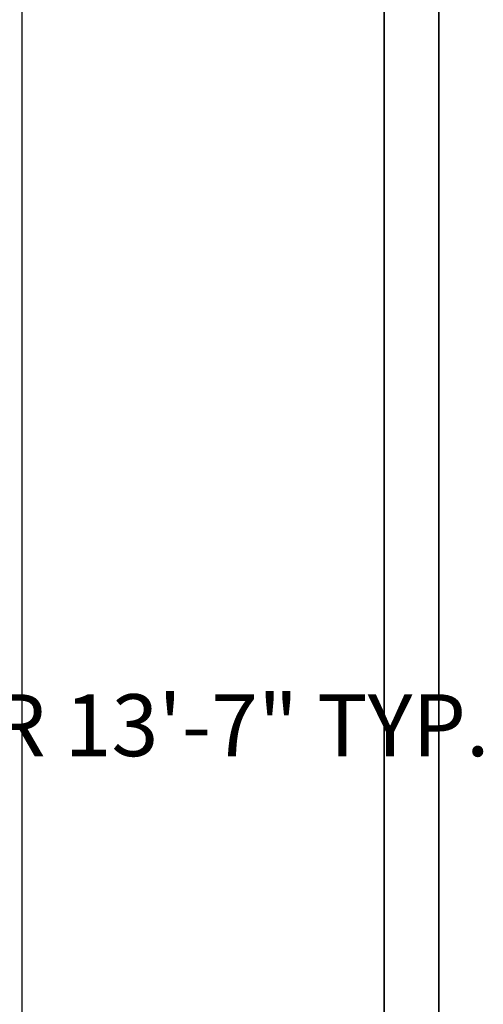
# Model space of a CAD drawing. Units: inches. Extents: x 1077 to 2505, y 1892 to 2728.
# Tile 10 of 26: x 1579 to 1655, y 2176 to 2338. Entities that reach past the tile are written whole.
import ezdxf

# ---------------------------------------------------------------- set-up
doc = ezdxf.new("R2010")
doc.units = ezdxf.units.IN
doc.linetypes.add('ACAD_ISO02W100', pattern=[15, 12, -3])
doc.layers.get('Defpoints').update_dxf_attribs({"color": 220, "linetype": 'ACAD_ISO02W100'})
doc.layers.add('A-ANNO-DIMS', color=2, linetype='Continuous', lineweight=18)
doc.layers.add('A-ANNO-TTLB', color=7, linetype='Continuous', lineweight=35)
doc.styles.get("Standard").update_dxf_attribs({"font": 'arial.ttf'})
doc.dimstyles.get("Standard").update_dxf_attribs({"dimtxt": 10.18, "dimasz": 0.18, "dimexe": 0.18, "dimexo": 0.0625, "dimgap": 0.09, "dimtad": 0, "dimtih": 1, "dimtoh": 1, "dimdec": 0, "dimzin": 0, "dimdsep": 46, "dimlunit": 3, "dimtxsty": 'Standard', "dimcen": 0.09, "dimadec": 0, "dimazin": 0, "dimtfac": 1, "dimtdec": 0, "dimtofl": 0, "dimtmove": 0, "dimatfit": 3, "dimfxl": 1, "dimtolj": 1, "dimtzin": 0, "dimarcsym": 0})

# ---------------------------------------------------------------- blocks, each defined once
blk = doc.blocks.new('*D14')
at = {"layer": 'A-ANNO-DIMS', "color": 0, "lineweight": -2, "transparency": 16777216}
for p, q in [((1555.59, 2651.66), (1579.43, 2651.66)), ((1579.25, 2651.48), (1579.25, 2375.3)), ((1579.25, 2088.54), (1579.25, 2364.72)), ((1555.59, 2088.36), (1579.43, 2088.36))]:
    blk.add_line(p, q, dxfattribs=at)
at = {"layer": 'A-ANNO-DIMS', "color": 0, "transparency": 16777216}
for points in [[(1579.22, 2651.48), (1579.28, 2651.48), (1579.25, 2651.66)], [(1579.22, 2088.54), (1579.28, 2088.54), (1579.25, 2088.36)]]:
    blk.add_solid(points, dxfattribs=at)
at = {"layer": 'Defpoints', "color": 0, "transparency": 16777216}
for p in [(1555.53, 2651.66), (1555.53, 2088.36), (1579.25, 2088.36)]:
    blk.add_point(p, dxfattribs=at)
at = {"layer": 'A-ANNO-DIMS', "color": 0, "transparency": 16777216, "insert": (1579.25, 2370.01), "char_height": 10.18, "attachment_point": 5}
blk.add_mtext('\\A1;46\'-11"', dxfattribs=at)
blk = doc.blocks.new('SHEET-FRAME-RESIDENTIAL')
for points in [[(0, 830.04), (543.52, 830.04), (543.52, 0), (0, 0)], [(9, 821.04), (534.52, 821.04), (534.52, 9), (9, 9)]]:
    blk.add_lwpolyline(points, close=True)
blk = doc.blocks.new('*D44')
at = {"layer": 'A-ANNO-DIMS', "color": 0, "lineweight": -2, "transparency": 16777216}
for p, q in [((1547.59, 2303.16), (1572.17, 2303.16)), ((1571.99, 2302.98), (1571.99, 2226.98)), ((1571.99, 2140.26), (1571.99, 2216.26)), ((1547.59, 2140.08), (1572.17, 2140.08))]:
    blk.add_line(p, q, dxfattribs=at)
at = {"layer": 'A-ANNO-DIMS', "color": 0, "transparency": 16777216}
for points in [[(1571.96, 2302.98), (1572.02, 2302.98), (1571.99, 2303.16)], [(1571.96, 2140.26), (1572.02, 2140.26), (1571.99, 2140.08)]]:
    blk.add_solid(points, dxfattribs=at)
at = {"layer": 'Defpoints', "color": 0, "transparency": 16777216}
for p in [(1547.53, 2303.16), (1571.99, 2303.16), (1547.53, 2140.08)]:
    blk.add_point(p, dxfattribs=at)
at = {"layer": 'A-ANNO-DIMS', "color": 0, "transparency": 16777216, "insert": (1571.99, 2221.62), "char_height": 10.18, "attachment_point": 5}
blk.add_mtext('\\A1;RETURN STAIR 13\'-7" TYP.', dxfattribs=at)

msp = doc.modelspace()

# ---------------------------------------------------------------- block references
at = {"layer": 'A-ANNO-TTLB'}
msp.add_blockref('SHEET-FRAME-RESIDENTIAL', (1104.25, 1892.27), dxfattribs=at)

# ---------------------------------------------------------------- dimensions: what is measured, and where the dimension line sits
at = {"layer": 'A-ANNO-DIMS'}
dim = msp.add_linear_dim(base=(1579.25, 2088.36), p1=(1555.53, 2651.66), p2=(1555.53, 2088.36), angle=90, dimstyle='Standard', override={"dimclrd": 0, "dimclre": 0, "dimclrt": 0}, dxfattribs=at)
dim.commit()
dim.dimension.update_dxf_attribs({"geometry": '*D14', "text_midpoint": (1579.25, 2370.01)})
dim = msp.add_linear_dim(base=(1571.99, 2303.16), p1=(1547.53, 2140.08), p2=(1547.53, 2303.16), angle=90, text='RETURN STAIR <> TYP.', dimstyle='Standard', override={"dimdec": 1, "dimlfac": 1, "dimrnd": 0, "dimzin": 1, "dimdsep": 46, "dimlunit": 4, "dimfrac": 2}, dxfattribs=at)
dim.commit()
dim.dimension.update_dxf_attribs({"geometry": '*D44', "text_midpoint": (1571.99, 2221.62)})

doc.saveas('drawing.dxf')
